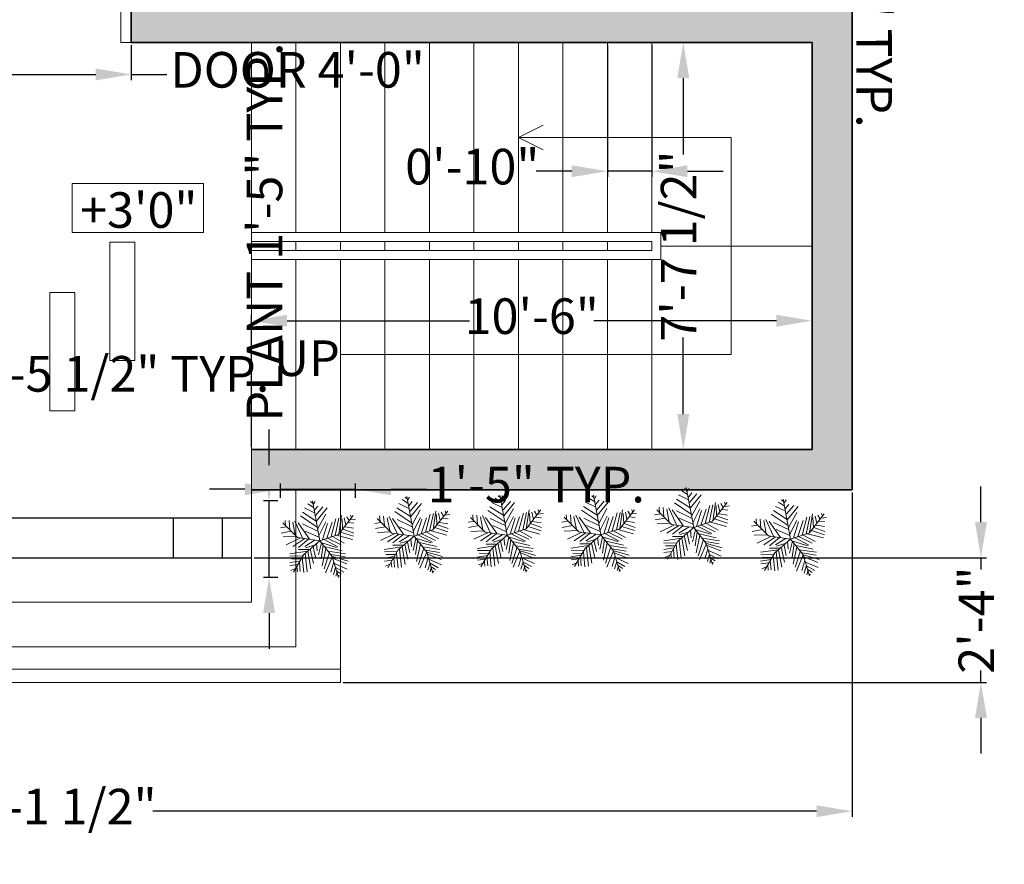
# Model space of a CAD drawing. Units: inches. Extents: x 2408 to 5087, y 2429 to 5085.
# Tile 7 of 12: x 2636 to 2858, y 2429 to 2619. Entities that reach past the tile are written whole.
import ezdxf

# ---------------------------------------------------------------- set-up
doc = ezdxf.new("R2010")
doc.units = ezdxf.units.IN
for name, color, linetype, lineweight in [('A-ANNO-DIMS', 2, 'Continuous', 18), ('A-ANNO-SYMB', 6, 'Continuous', 18), ('A-DOOR', 3, 'Continuous', 18), ('A-FLOR', 7, 'Continuous', 25), ('A-FLOR-STRS', 7, 'Continuous', 18), ('A-WALL', 7, 'Continuous', 35), ('A-WALL-PATT', 252, 'Continuous', 13), ('L-HRDS-PVMT', 8, 'Continuous', 18), ('L-PLNT', 3, 'Continuous', 13)]:
    doc.layers.add(name, color=color, linetype=linetype, lineweight=lineweight)
doc.styles.get("Standard").update_dxf_attribs({"font": 'arial.ttf'})
doc.dimstyles.new('ISO-25', dxfattribs={"dimtxt": 8, "dimasz": 8, "dimexe": 1.25, "dimexo": 0.625, "dimtad": 0, "dimdec": 1, "dimlunit": 4, "dimtxsty": 'Standard', "dimcen": 2.5, "dimadec": 0, "dimazin": 0, "dimtfac": 1, "dimtdec": 1, "dimtmove": 0, "dimatfit": 3, "dimfxl": 1, "dimarcsym": 0})

# ---------------------------------------------------------------- blocks, each defined once
blk = doc.blocks.new('door')
blk.add_lwpolyline([(2353.25, 2862.23), (2353.25, 2898.06), (2351.47, 2898.06), (2351.47, 2862.23), (2353.25, 2862.23)])
blk.add_arc((2353.25, 2862.23), 35.83, 90, 180)
blk = doc.blocks.new('tree')
for p, q in [((2943.9, 2571.4), (2933.4, 2628.4)), ((2936.6, 2611.1), (2922.1, 2618.1)), ((2935.2, 2618.6), (2926.8, 2624.1)), ((2933.7, 2625.1), (2930.8, 2627.4)), ((2934.8, 2623.2), (2937.4, 2627.4)), ((2936.3, 2614.8), (2941.3, 2620.9)), ((2938.1, 2607.4), (2948.6, 2619.5)), ((2938.8, 2599), (2954.4, 2618.1)), ((2895.3, 2592.5), (2894.6, 2600.4)), ((2900.4, 2600), (2901.5, 2587)), ((2940.3, 2590.7), (2916.3, 2606.9)), ((2938.8, 2599.5), (2919.2, 2612.1)), ((2941, 2587.9), (2952.6, 2609.3)), ((2960.2, 2577.2), (2967.1, 2602.8)), ((2966, 2578.6), (2971.4, 2603.7)), ((2970.9, 2580.4), (2991.9, 2607.4)), ((2971, 2580.5), (2975, 2607.4)), ((2975.8, 2602.3), (2976.5, 2587.9)), ((2979, 2604.2), (2981.2, 2593.9)), ((2982.6, 2605.6), (2985.9, 2600)), ((2987.7, 2601.4), (2995, 2602.3)), ((2988.1, 2607.9), (2989.2, 2604.2)), ((2896.4, 2591.2), (2888.1, 2589.8)), ((2912.4, 2575.9), (2891.4, 2596.9)), ((2905.5, 2597.7), (2909.1, 2579.1)), ((2908.4, 2599.5), (2919.6, 2575.4)), ((2929.4, 2573.5), (2913.1, 2596.7)), ((2919.6, 2595.3), (2941, 2585.1)), ((2942.8, 2578.2), (2952.9, 2598.1)), ((2947.9, 2573), (2955.1, 2595.8)), ((2954, 2574.9), (2961.6, 2597.7)), ((2977.2, 2587.9), (2992.8, 2582.3)), ((2980.1, 2591.2), (2992.1, 2589.3)), ((2984.4, 2597.2), (2992.8, 2596.3)), ((2903.3, 2585.1), (2888.8, 2582.3)), ((2910.5, 2577.7), (2891.7, 2576.8)), ((2915.6, 2574.9), (2896.1, 2565.6)), ((2922.5, 2574.4), (2905.8, 2563.3)), ((2943.9, 2571.4), (2912.4, 2575.9)), ((2927.9, 2573.5), (2913.8, 2561.9)), ((2937.4, 2572.6), (2922.5, 2563.3)), ((2923.2, 2585.1), (2942.8, 2576.3)), ((2943.9, 2571.4), (2970.9, 2580.4)), ((2950.4, 2573), (2970, 2562.8)), ((2955.1, 2574.9), (2974.7, 2565.6)), ((2962, 2577.2), (2979, 2567.9)), ((2968.1, 2579.1), (2990.6, 2573)), ((2973.6, 2583.7), (2992.1, 2577.7)), ((2928.7, 2558.6), (2913.8, 2558.6)), ((2943.9, 2571.4), (2921.4, 2551.9)), ((2937.4, 2565.6), (2923.9, 2561.4)), ((2930.5, 2560), (2935.2, 2538.7)), ((2934.5, 2562.8), (2937.7, 2548)), ((2939.2, 2567.9), (2940.3, 2556.8)), ((2946.4, 2568.4), (2942.4, 2551.2)), ((2943.9, 2571.4), (2961.9, 2548.9)), ((2945.7, 2568.9), (2968.1, 2561.9)), ((2948.9, 2565.1), (2946, 2545.6)), ((2952.9, 2560), (2947.5, 2535.4)), ((2951.5, 2562.4), (2976.1, 2556.8)), ((2926.5, 2556.3), (2901.1, 2552.6)), ((2919.6, 2549.8), (2901.5, 2549.4)), ((2917.1, 2545.2), (2903.7, 2545.6)), ((2921.4, 2551.9), (2906.4, 2526.4)), ((2918.9, 2547.5), (2921.1, 2526.1)), ((2923.2, 2553.1), (2926.1, 2527.1)), ((2926.8, 2556.3), (2931.2, 2531.2)), ((2958, 2554.5), (2950.4, 2531.2)), ((2962, 2548.9), (2952.2, 2525.7)), ((2956.2, 2556.3), (2980.8, 2552.6)), ((2960.2, 2551.7), (2980.1, 2548.4)), ((2961.9, 2548.9), (2970.9, 2518.9)), ((2962.3, 2548.9), (2984.4, 2542.4)), ((2963.1, 2546.1), (2982.6, 2538.2)), ((2915.6, 2542.4), (2901.1, 2540.1)), ((2913.1, 2537.3), (2901.5, 2535.9)), ((2909.5, 2531.7), (2902.9, 2528.9)), ((2911.3, 2534.5), (2912, 2527.1)), ((2914.9, 2540.5), (2916, 2527.5)), ((2964.2, 2541), (2959.8, 2526.6)), ((2966.7, 2533.6), (2963.4, 2522.9)), ((2965.2, 2538.7), (2983, 2530.8)), ((2966.7, 2533.1), (2978.3, 2526.6)), ((2968.5, 2525.7), (2967.1, 2520.6)), ((2968.5, 2528), (2974.7, 2523.8)), ((2970.7, 2521.5), (2972.1, 2520.6))]:
    blk.add_line(p, q)
blk = doc.blocks.new('LEVEL-TAG-FRAME')
blk.add_line((29.47, 11), (29.47, 0))
blk.add_lwpolyline([(29.47, 0), (0, 0), (0, 11), (29.47, 11)])
blk = doc.blocks.new('PORTICO-PAVER')
blk.add_lwpolyline([(0, 26.64), (5.57, 26.64), (5.57, 0), (0, 0)], close=True)
blk = doc.blocks.new('*D27')
at = {"layer": 'A-ANNO-DIMS', "color": 0, "lineweight": -2, "transparency": 16777216}
for p, q in [((2612.36, 2568.68), (2612.36, 2576.68)), ((2608.98, 2568.68), (2613.61, 2568.68)), ((2612.36, 2550.04), (2612.36, 2560.68)), ((2608.98, 2542.04), (2613.61, 2542.04))]:
    blk.add_line(p, q, dxfattribs=at)
at = {"layer": 'A-ANNO-DIMS', "color": 0, "transparency": 16777216}
for points in [[(2611.02, 2560.68), (2613.69, 2560.68), (2612.36, 2568.68)], [(2611.02, 2550.04), (2613.69, 2550.04), (2612.36, 2542.04)]]:
    blk.add_solid(points, dxfattribs=at)
at = {"layer": 'Defpoints', "color": 0, "transparency": 16777216}
for p in [(2608.36, 2568.68), (2612.36, 2568.68), (2608.36, 2542.04)]:
    blk.add_point(p, dxfattribs=at)
at = {"layer": 'A-ANNO-DIMS', "color": 0, "transparency": 16777216, "insert": (2612.36, 2631.3), "char_height": 8, "attachment_point": 5, "rotation": 90}
blk.add_mtext('PAVER 2\'-2 1/2" TYP.', dxfattribs=at)
blk = doc.blocks.new('*D28')
at = {"layer": 'A-ANNO-DIMS', "color": 0, "lineweight": -2, "transparency": 16777216}
for p, q in [((2602.79, 2541.41), (2602.79, 2536.79)), ((2608.36, 2541.41), (2608.36, 2536.79)), ((2594.79, 2538.04), (2586.79, 2538.04)), ((2602.79, 2538.04), (2608.36, 2538.04)), ((2616.36, 2538.04), (2624.36, 2538.04))]:
    blk.add_line(p, q, dxfattribs=at)
at = {"layer": 'A-ANNO-DIMS', "color": 0, "transparency": 16777216}
for points in [[(2594.79, 2539.38), (2594.79, 2536.71), (2602.79, 2538.04)], [(2616.36, 2539.38), (2616.36, 2536.71), (2608.36, 2538.04)]]:
    blk.add_solid(points, dxfattribs=at)
at = {"layer": 'Defpoints', "color": 0, "transparency": 16777216}
for p in [(2602.79, 2542.04), (2608.36, 2542.04), (2608.36, 2538.04)]:
    blk.add_point(p, dxfattribs=at)
at = {"layer": 'A-ANNO-DIMS', "color": 0, "transparency": 16777216, "insert": (2658.69, 2538.04), "char_height": 8, "attachment_point": 5}
blk.add_mtext('0\'-5 1/2" TYP.', dxfattribs=at)
blk = doc.blocks.new('*D31')
at = {"layer": 'A-ANNO-DIMS', "color": 0, "lineweight": -2, "transparency": 16777216}
for p, q in [((2692.46, 2518.56), (2692.46, 2526.56)), ((2694.42, 2510.56), (2691.21, 2510.56)), ((2692.46, 2493.32), (2692.46, 2510.56)), ((2694.42, 2493.32), (2691.21, 2493.32)), ((2692.46, 2485.32), (2692.46, 2477.32))]:
    blk.add_line(p, q, dxfattribs=at)
at = {"layer": 'A-ANNO-DIMS', "color": 0, "transparency": 16777216}
for points in [[(2691.12, 2518.56), (2693.79, 2518.56), (2692.46, 2510.56)], [(2691.12, 2485.32), (2693.79, 2485.32), (2692.46, 2493.32)]]:
    blk.add_solid(points, dxfattribs=at)
at = {"layer": 'Defpoints', "color": 0, "transparency": 16777216}
for p in [(2692.46, 2510.56), (2695.04, 2510.56), (2695.04, 2493.32)]:
    blk.add_point(p, dxfattribs=at)
at = {"layer": 'A-ANNO-DIMS', "color": 0, "transparency": 16777216, "insert": (2692.46, 2570.93), "char_height": 8, "attachment_point": 5, "rotation": 90}
blk.add_mtext('PLANT 1\'-5" TYP.', dxfattribs=at)
blk = doc.blocks.new('*D32')
at = {"layer": 'A-ANNO-DIMS', "color": 0, "lineweight": -2, "transparency": 16777216}
for p, q in [((2695.04, 2511.18), (2695.04, 2514.4)), ((2711.87, 2511.18), (2711.87, 2514.4)), ((2687.04, 2513.15), (2679.04, 2513.15)), ((2695.04, 2513.15), (2711.87, 2513.15)), ((2719.87, 2513.15), (2727.87, 2513.15))]:
    blk.add_line(p, q, dxfattribs=at)
at = {"layer": 'A-ANNO-DIMS', "color": 0, "transparency": 16777216}
for points in [[(2687.04, 2514.48), (2687.04, 2511.81), (2695.04, 2513.15)], [(2719.87, 2514.48), (2719.87, 2511.81), (2711.87, 2513.15)]]:
    blk.add_solid(points, dxfattribs=at)
at = {"layer": 'Defpoints', "color": 0, "transparency": 16777216}
for p in [(2711.87, 2513.15), (2695.04, 2510.56), (2711.87, 2510.56)]:
    blk.add_point(p, dxfattribs=at)
at = {"layer": 'A-ANNO-DIMS', "color": 0, "transparency": 16777216, "insert": (2752.5, 2513.15), "char_height": 8, "attachment_point": 5}
blk.add_mtext('1\'-5" TYP.', dxfattribs=at)
blk = doc.blocks.new('*D39')
at = {"layer": 'A-ANNO-DIMS', "color": 0, "lineweight": -2, "transparency": 16777216}
for p, q in [((2613.46, 2612.93), (2613.46, 2605.1)), ((2661.49, 2612.93), (2661.49, 2605.1)), ((2621.46, 2606.35), (2653.49, 2606.35)), ((2661.49, 2606.35), (2669.49, 2606.35))]:
    blk.add_line(p, q, dxfattribs=at)
at = {"layer": 'A-ANNO-DIMS', "color": 0, "transparency": 16777216}
for points in [[(2621.46, 2607.68), (2621.46, 2605.02), (2613.46, 2606.35)], [(2653.49, 2607.68), (2653.49, 2605.02), (2661.49, 2606.35)]]:
    blk.add_solid(points, dxfattribs=at)
at = {"layer": 'Defpoints', "color": 0, "transparency": 16777216}
for p in [(2613.46, 2613.55), (2661.49, 2613.55), (2661.49, 2606.35)]:
    blk.add_point(p, dxfattribs=at)
at = {"layer": 'A-ANNO-DIMS', "color": 0, "transparency": 16777216, "insert": (2698.87, 2606.35), "char_height": 8, "attachment_point": 5}
blk.add_mtext('DOOR 4\'-0"', dxfattribs=at)
blk = doc.blocks.new('*D40')
at = {"layer": 'A-ANNO-DIMS', "color": 0, "lineweight": -2, "transparency": 16777216}
for p, q in [((2662.12, 2661.59), (2669.95, 2661.59)), ((2668.7, 2653.59), (2668.7, 2648.99)), ((2668.7, 2621.55), (2668.7, 2626.15)), ((2662.12, 2613.55), (2669.95, 2613.55))]:
    blk.add_line(p, q, dxfattribs=at)
at = {"layer": 'A-ANNO-DIMS', "color": 0, "transparency": 16777216}
for points in [[(2667.37, 2653.59), (2670.03, 2653.59), (2668.7, 2661.59)], [(2667.37, 2621.55), (2670.03, 2621.55), (2668.7, 2613.55)]]:
    blk.add_solid(points, dxfattribs=at)
at = {"layer": 'Defpoints', "color": 0, "transparency": 16777216}
for p in [(2661.49, 2661.59), (2668.7, 2661.59), (2661.49, 2613.55)]:
    blk.add_point(p, dxfattribs=at)
at = {"layer": 'A-ANNO-DIMS', "color": 0, "transparency": 16777216, "insert": (2668.7, 2637.57), "char_height": 8, "attachment_point": 5, "rotation": 90}
blk.add_mtext('4\'-0"', dxfattribs=at)
blk = doc.blocks.new('*D43')
at = {"layer": 'A-ANNO-DIMS', "color": 0, "lineweight": -2, "transparency": 16777216}
for p, q in [((2814.95, 2783.84), (2827.96, 2783.89)), ((2826.75, 2775.89), (2827.01, 2709.32)), ((2815.28, 2701.27), (2828.29, 2701.33)), ((2827.04, 2701.32), (2827.07, 2693.32))]:
    blk.add_line(p, q, dxfattribs=at)
at = {"layer": 'A-ANNO-DIMS', "color": 0, "transparency": 16777216}
for points in [[(2828.08, 2775.89), (2825.41, 2775.88), (2826.71, 2783.89)], [(2828.34, 2709.33), (2825.68, 2709.32), (2827.04, 2701.32)]]:
    blk.add_solid(points, dxfattribs=at)
at = {"layer": 'Defpoints', "color": 0, "transparency": 16777216}
for p in [(2814.33, 2783.84), (2814.66, 2701.27), (2827.04, 2701.32)]:
    blk.add_point(p, dxfattribs=at)
at = {"layer": 'A-ANNO-DIMS', "color": 0, "transparency": 16777216, "insert": (2827.27, 2643.02), "char_height": 8, "attachment_point": 5, "rotation": 270.2276}
blk.add_mtext('BED 6\'-10 1/2" TYP.', dxfattribs=at)
blk = doc.blocks.new('*D64')
at = {"layer": 'A-ANNO-DIMS', "color": 0, "lineweight": -2, "transparency": 16777216}
for p, q in [((2852.44, 2505.75), (2852.44, 2513.75)), ((2689.12, 2497.75), (2853.69, 2497.75)), ((2852.44, 2497.75), (2852.44, 2495.08)), ((2852.44, 2469.75), (2852.44, 2472.42)), ((2709.12, 2469.75), (2853.69, 2469.75)), ((2852.44, 2461.75), (2852.44, 2453.75))]:
    blk.add_line(p, q, dxfattribs=at)
at = {"layer": 'A-ANNO-DIMS', "color": 0, "transparency": 16777216}
for points in [[(2851.11, 2505.75), (2853.78, 2505.75), (2852.44, 2497.75)], [(2851.11, 2461.75), (2853.78, 2461.75), (2852.44, 2469.75)]]:
    blk.add_solid(points, dxfattribs=at)
at = {"layer": 'Defpoints', "color": 0, "transparency": 16777216}
for p in [(2688.49, 2497.75), (2852.44, 2497.75), (2708.49, 2469.75)]:
    blk.add_point(p, dxfattribs=at)
at = {"layer": 'A-ANNO-DIMS', "color": 0, "transparency": 16777216, "insert": (2852.44, 2483.75), "char_height": 8, "attachment_point": 5, "rotation": 90}
blk.add_mtext('2\'-4"', dxfattribs=at)
blk = doc.blocks.new('*D65')
at = {"layer": 'A-ANNO-DIMS', "color": 0, "lineweight": -2, "transparency": 16777216}
for p, q in [((2823.49, 2512.43), (2823.49, 2439.55)), ((2461.88, 2469.13), (2461.88, 2439.55)), ((2469.88, 2440.8), (2619, 2440.8)), ((2815.49, 2440.8), (2666.37, 2440.8))]:
    blk.add_line(p, q, dxfattribs=at)
at = {"layer": 'A-ANNO-DIMS', "color": 0, "transparency": 16777216}
for points in [[(2469.88, 2442.13), (2469.88, 2439.47), (2461.88, 2440.8)], [(2815.49, 2442.13), (2815.49, 2439.47), (2823.49, 2440.8)]]:
    blk.add_solid(points, dxfattribs=at)
at = {"layer": 'Defpoints', "color": 0, "transparency": 16777216}
for p in [(2823.49, 2513.05), (2461.88, 2469.75), (2823.49, 2440.8)]:
    blk.add_point(p, dxfattribs=at)
at = {"layer": 'A-ANNO-DIMS', "color": 0, "transparency": 16777216, "insert": (2642.69, 2440.8), "char_height": 8, "attachment_point": 5}
blk.add_mtext('30\'-1 1/2"', dxfattribs=at)
blk = doc.blocks.new('*D67')
at = {"layer": 'A-ANNO-DIMS', "color": 0, "lineweight": -2, "transparency": 16777216}
for p, q in [((2688.49, 2522.68), (2688.49, 2552.25)), ((2814.49, 2522.68), (2814.49, 2552.25)), ((2696.49, 2551), (2737.5, 2551)), ((2806.49, 2551), (2765.48, 2551))]:
    blk.add_line(p, q, dxfattribs=at)
at = {"layer": 'A-ANNO-DIMS', "color": 0, "transparency": 16777216}
for points in [[(2696.49, 2552.34), (2696.49, 2549.67), (2688.49, 2551)], [(2806.49, 2552.34), (2806.49, 2549.67), (2814.49, 2551)]]:
    blk.add_solid(points, dxfattribs=at)
at = {"layer": 'Defpoints', "color": 0, "transparency": 16777216}
for p in [(2814.49, 2551), (2688.49, 2522.05), (2814.49, 2522.05)]:
    blk.add_point(p, dxfattribs=at)
at = {"layer": 'A-ANNO-DIMS', "color": 0, "transparency": 16777216, "insert": (2751.49, 2551), "char_height": 8, "attachment_point": 5}
blk.add_mtext('10\'-6"', dxfattribs=at)
blk = doc.blocks.new('*D68')
at = {"layer": 'A-ANNO-DIMS', "color": 0, "lineweight": -2, "transparency": 16777216}
for p, q in [((2768.49, 2612.93), (2768.49, 2583.35)), ((2778.49, 2612.93), (2778.49, 2583.35)), ((2760.49, 2584.6), (2752.49, 2584.6)), ((2778.49, 2584.6), (2768.49, 2584.6)), ((2786.49, 2584.6), (2794.49, 2584.6))]:
    blk.add_line(p, q, dxfattribs=at)
at = {"layer": 'A-ANNO-DIMS', "color": 0, "transparency": 16777216}
for points in [[(2760.49, 2585.94), (2760.49, 2583.27), (2768.49, 2584.6)], [(2786.49, 2585.94), (2786.49, 2583.27), (2778.49, 2584.6)]]:
    blk.add_solid(points, dxfattribs=at)
at = {"layer": 'Defpoints', "color": 0, "transparency": 16777216}
for p in [(2768.49, 2613.55), (2778.49, 2613.55), (2768.49, 2584.6)]:
    blk.add_point(p, dxfattribs=at)
at = {"layer": 'A-ANNO-DIMS', "color": 0, "transparency": 16777216, "insert": (2738.13, 2584.6), "char_height": 8, "attachment_point": 5}
blk.add_mtext('0\'-10"', dxfattribs=at)
blk = doc.blocks.new('*D69')
at = {"layer": 'A-ANNO-DIMS', "color": 0, "lineweight": -2, "transparency": 16777216}
for p, q in [((2813.87, 2613.55), (2784.29, 2613.55)), ((2785.54, 2605.55), (2785.54, 2588.35)), ((2785.54, 2530.05), (2785.54, 2547.26)), ((2813.87, 2522.05), (2784.29, 2522.05))]:
    blk.add_line(p, q, dxfattribs=at)
at = {"layer": 'A-ANNO-DIMS', "color": 0, "transparency": 16777216}
for points in [[(2784.21, 2605.55), (2786.88, 2605.55), (2785.54, 2613.55)], [(2784.21, 2530.05), (2786.88, 2530.05), (2785.54, 2522.05)]]:
    blk.add_solid(points, dxfattribs=at)
at = {"layer": 'Defpoints', "color": 0, "transparency": 16777216}
for p in [(2785.54, 2613.55), (2814.49, 2613.55), (2814.49, 2522.05)]:
    blk.add_point(p, dxfattribs=at)
at = {"layer": 'A-ANNO-DIMS', "color": 0, "transparency": 16777216, "insert": (2785.54, 2567.8), "char_height": 8, "attachment_point": 5, "rotation": 90}
blk.add_mtext('7\'-7 1/2"', dxfattribs=at)

msp = doc.modelspace()

# ---------------------------------------------------------------- hatches: boundary and pattern name
at = {"layer": 'A-WALL-PATT'}
h = msp.add_hatch(color=256, dxfattribs=at)
h.dxf.hatch_style = 1
h.paths.add_polyline_path([(2493.49, 2613.55), (2523.49, 2613.55), (2523.49, 2622.55), (2493.49, 2622.55), (2493.49, 2714.8), (2484.49, 2714.8), (2484.49, 2497.75), (2493.49, 2497.75)])
h.paths.add_polyline_path([(2613.49, 2615.42), (2613.49, 2622.55), (2583.49, 2622.55), (2583.49, 2613.55), (2613.46, 2613.55, -0.009707)])
h.paths.add_polyline_path([(2823.49, 2634.55), (2814.49, 2634.55), (2814.49, 2622.55), (2694.49, 2622.55), (2694.49, 2670.55), (2706.49, 2670.55), (2706.49, 2675.05), (2694.49, 2675.05), (2694.49, 2750.05), (2685.49, 2750.05), (2685.49, 2622.55), (2661.49, 2622.55), (2661.49, 2613.55), (2814.49, 2613.55), (2814.49, 2522.05), (2688.49, 2522.05), (2688.49, 2513.05), (2823.49, 2513.05)])
h.paths.add_polyline_path([(2823.49, 2837.05), (2814.49, 2837.05), (2814.49, 2819.05), (2685.49, 2819.05), (2685.49, 2786.05), (2694.49, 2786.05), (2694.49, 2810.05), (2814.49, 2810.05), (2814.49, 2772.55), (2823.49, 2772.55)])
h.paths.add_polyline_path([(2694.49, 2964.55), (2595.49, 2964.55), (2595.49, 3008.05), (2601.49, 3008.05), (2601.49, 3017.05), (2484.49, 3017.05), (2484.49, 2972.05), (2493.49, 2972.05), (2493.49, 3008.05), (2586.49, 3008.05), (2586.49, 2955.55), (2685.49, 2955.55), (2685.49, 2854.87), (2694.49, 2854.87)])
h.paths.add_polyline_path([(2493.49, 2867.05), (2595.49, 2867.05), (2595.49, 2876.05), (2493.49, 2876.05), (2493.49, 2912.05), (2484.49, 2912.05), (2484.49, 2774.8), (2493.49, 2774.8)])
h.paths.add_polyline_path([(2595.49, 2814.55), (2493.49, 2814.55), (2493.49, 2810.05), (2595.49, 2810.05)], flags=17)
h.paths.add_polyline_path([(2724.49, 3017.05), (2625.49, 3017.05), (2625.49, 3008.05), (2685.49, 3008.05), (2685.49, 2994.55), (2694.49, 2994.55), (2694.49, 3008.05), (2724.49, 3008.05)])
h.paths.add_polyline_path([(2823.49, 3017.05), (2784.49, 3017.05), (2784.49, 3008.05), (2814.49, 3008.05), (2814.49, 2913.55), (2814.56, 2897.05), (2823.49, 2897.05)])
h.paths.add_polyline_path([(2823.49, 2712.55), (2814.61, 2712.55), (2814.66, 2701.27), (2814.49, 2701.27), (2814.49, 2675.05), (2740.99, 2675.05), (2740.99, 2687.05), (2736.49, 2687.05), (2736.49, 2670.55), (2814.49, 2670.55), (2814.49, 2658.55), (2823.49, 2658.55)], flags=17)

# ---------------------------------------------------------------- linework, layer by layer
at = {"layer": 'A-ANNO-SYMB'}
for p, q in [((2748.49, 2592.18), (2754.06, 2594.96)), ((2748.49, 2592.18), (2796.29, 2592.18)), ((2748.49, 2592.18), (2754.06, 2589.4)), ((2796.29, 2543.43), (2796.29, 2592.18)), ((2708.49, 2543.43), (2796.29, 2543.43))]:
    msp.add_line(p, q, dxfattribs=at)
at = {"layer": 'A-FLOR'}
for p, q in [((2493.49, 2506.75), (2688.49, 2506.75)), ((2670.94, 2506.75), (2670.94, 2497.75)), ((2681.89, 2506.75), (2681.89, 2497.75)), ((2484.49, 2497.75), (2688.49, 2497.75))]:
    msp.add_line(p, q, dxfattribs=at)
at = {"layer": 'A-FLOR-STRS'}
for p, q in [((2688.49, 2487.75), (2688.49, 2613.55)), ((2698.49, 2570.8), (2698.49, 2613.55)), ((2708.49, 2570.8), (2708.49, 2613.55)), ((2718.49, 2570.8), (2718.49, 2613.55)), ((2728.49, 2570.8), (2728.49, 2613.55)), ((2738.49, 2570.8), (2738.49, 2613.55)), ((2748.49, 2570.8), (2748.49, 2613.55)), ((2758.49, 2570.8), (2758.49, 2613.55)), ((2768.49, 2570.8), (2768.49, 2613.55)), ((2778.49, 2570.8), (2778.49, 2613.55)), ((2780.49, 2570.8), (2688.49, 2570.8)), ((2780.49, 2564.8), (2780.49, 2570.8)), ((2778.49, 2568.8), (2688.49, 2568.8)), ((2698.49, 2566.8), (2698.49, 2568.8)), ((2708.49, 2566.8), (2708.49, 2568.8)), ((2718.49, 2566.8), (2718.49, 2568.8)), ((2728.49, 2566.8), (2728.49, 2568.8)), ((2738.49, 2566.8), (2738.49, 2568.8)), ((2748.49, 2566.8), (2748.49, 2568.8)), ((2758.49, 2566.8), (2758.49, 2568.8)), ((2768.49, 2566.8), (2768.49, 2568.8)), ((2778.49, 2566.8), (2778.49, 2568.8)), ((2780.49, 2567.8), (2814.49, 2567.8)), ((2778.49, 2566.8), (2688.49, 2566.8)), ((2780.49, 2564.8), (2688.49, 2564.8)), ((2698.49, 2522.05), (2698.49, 2564.8)), ((2708.49, 2522.05), (2708.49, 2564.8)), ((2718.49, 2522.05), (2718.49, 2564.8)), ((2728.49, 2522.05), (2728.49, 2564.8)), ((2738.49, 2522.05), (2738.49, 2564.8)), ((2748.49, 2522.05), (2748.49, 2564.8)), ((2758.49, 2522.05), (2758.49, 2564.8)), ((2768.49, 2522.05), (2768.49, 2564.8)), ((2778.49, 2522.05), (2778.49, 2564.8)), ((2698.49, 2477.75), (2698.49, 2513.05)), ((2708.49, 2469.75), (2708.49, 2513.05)), ((2476.42, 2487.75), (2688.49, 2487.75)), ((2468.34, 2477.75), (2698.49, 2477.75)), ((2464.3, 2472.75), (2708.49, 2472.75)), ((2461.88, 2469.75), (2708.49, 2469.75))]:
    msp.add_line(p, q, dxfattribs=at)
at = {"layer": 'A-WALL'}
for p, q in [((2823.49, 2513.05), (2823.49, 3017.05)), ((2661.49, 2622.55), (2661.49, 2613.55)), ((2814.49, 2613.55), (2661.49, 2613.55)), ((2814.49, 2522.05), (2814.49, 2613.55)), ((2814.49, 2522.05), (2688.49, 2522.05)), ((2823.49, 2513.05), (2688.49, 2513.05))]:
    msp.add_line(p, q, dxfattribs=at)

# ---------------------------------------------------------------- block references
at = {"layer": 'A-ANNO-SYMB'}
msp.add_blockref('LEVEL-TAG-FRAME', (2648.23, 2570.85), dxfattribs=at)
at = {"layer": 'A-DOOR', "xscale": 1.340790722123845, "yscale": 1.340790722123845, "zscale": 1.340790722123845}
msp.add_blockref('door', (-493.72, -1224.1), dxfattribs=at)
at = {"layer": 'L-HRDS-PVMT'}
for p in [(2656.7, 2542.04), (2643.22, 2530.73)]:
    msp.add_blockref('PORTICO-PAVER', p, dxfattribs=at)
at = {"layer": 'L-PLNT', "xscale": 0.1574495788251676, "yscale": 0.1574495788251676, "zscale": 0.1574495788251676}
for p in [(2261.53, 2097.71), (2282.47, 2097.95), (2303.51, 2098), (2324.37, 2099.66), (2240.32, 2096.72), (2346.16, 2097.08)]:
    msp.add_blockref('tree', p, dxfattribs=at)

# ---------------------------------------------------------------- texts
at = {"layer": 'A-ANNO-SYMB', "char_height": 8, "attachment_point": 1}
for s, width, insert in [('\\pxqc;+3\'0"', 102.8772, (2611.74, 2579.88)), ('\\pxqc;UP', 24.0903, (2688.92, 2546.59))]:
    msp.add_mtext_dynamic_manual_height_columns(s, width=width, gutter_width=12.5, heights=[0], dxfattribs=dict(at, insert=insert))

# ---------------------------------------------------------------- dimensions: what is measured, and where the dimension line sits
at = {"layer": 'A-ANNO-DIMS'}
for base, p1, p2, angle, text, picture, middle in [((2827.04, 2701.32), (2814.33, 2783.84), (2814.66, 2701.27), 270.2276, 'BED <> TYP.', '*D43', (2827.27, 2643.02)), ((2612.36, 2568.68), (2608.36, 2542.04), (2608.36, 2568.68), 90, 'PAVER <> TYP.', '*D27', (2612.36, 2631.3)), ((2692.46, 2510.56), (2695.04, 2493.32), (2695.04, 2510.56), 90, 'PLANT <> TYP.', '*D31', (2692.46, 2570.93))]:
    dim = msp.add_linear_dim(base=base, p1=p1, p2=p2, angle=angle, text=text, dimstyle='ISO-25', override={"dimdec": 1, "dimlfac": 1, "dimrnd": 0, "dimzin": 1, "dimdsep": 46, "dimlunit": 4, "dimfrac": 2}, dxfattribs=at)
    dim.commit()
    dim.dimension.update_dxf_attribs({"geometry": picture, "text_midpoint": middle})
for base, p1, p2, angle, picture, middle in [((2668.7, 2661.59), (2661.49, 2613.55), (2661.49, 2661.59), 90, '*D40', (2668.7, 2637.57)), ((2768.49, 2584.6), (2778.49, 2613.55), (2768.49, 2613.55), 180, '*D68', (2738.13, 2584.6)), ((2785.54, 2613.55), (2814.49, 2522.05), (2814.49, 2613.55), 90, '*D69', (2785.54, 2567.8)), ((2852.44, 2497.75), (2708.49, 2469.75), (2688.49, 2497.75), 90, '*D64', (2852.44, 2483.75))]:
    dim = msp.add_linear_dim(base=base, p1=p1, p2=p2, angle=angle, dimstyle='ISO-25', override={"dimdec": 1, "dimlfac": 1, "dimrnd": 0, "dimzin": 1, "dimdsep": 46, "dimlunit": 4, "dimfrac": 2}, dxfattribs=at)
    dim.commit()
    dim.dimension.update_dxf_attribs({"geometry": picture, "text_midpoint": middle})
for base, p1, p2, text, picture, middle in [((2661.49, 2606.35), (2613.46, 2613.55), (2661.49, 2613.55), 'DOOR <>', '*D39', (2698.87, 2606.35)), ((2608.36, 2538.04), (2602.79, 2542.04), (2608.36, 2542.04), '<> TYP.', '*D28', (2658.69, 2538.04)), ((2711.87, 2513.15), (2695.04, 2510.56), (2711.87, 2510.56), '<> TYP.', '*D32', (2752.5, 2513.15))]:
    dim = msp.add_linear_dim(base=base, p1=p1, p2=p2, text=text, dimstyle='ISO-25', override={"dimdec": 1, "dimlfac": 1, "dimrnd": 0, "dimzin": 1, "dimdsep": 46, "dimlunit": 4, "dimfrac": 2}, dxfattribs=at)
    dim.commit()
    dim.dimension.update_dxf_attribs({"geometry": picture, "text_midpoint": middle})
for base, p1, p2, picture, middle in [((2814.49, 2551), (2688.49, 2522.05), (2814.49, 2522.05), '*D67', (2751.49, 2551)), ((2823.49, 2440.8), (2461.88, 2469.75), (2823.49, 2513.05), '*D65', (2642.69, 2440.8))]:
    dim = msp.add_linear_dim(base=base, p1=p1, p2=p2, dimstyle='ISO-25', override={"dimdec": 1, "dimlfac": 1, "dimrnd": 0, "dimzin": 1, "dimdsep": 46, "dimlunit": 4, "dimfrac": 2}, dxfattribs=at)
    dim.commit()
    dim.dimension.update_dxf_attribs({"geometry": picture, "text_midpoint": middle})

doc.saveas('drawing.dxf')
